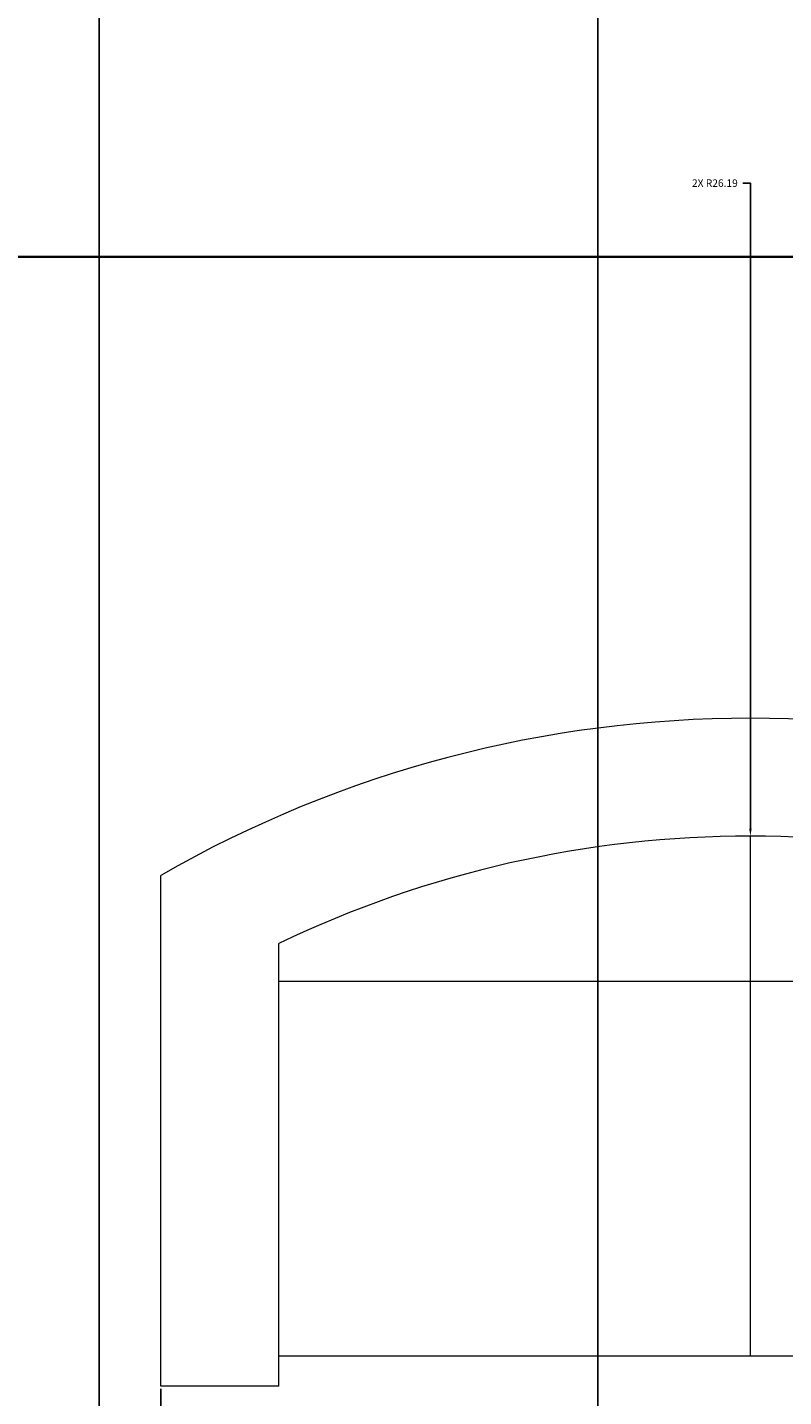
# Model space of a CAD drawing. Units: feet. Extents: x 1654 to 2985, y 1348 to 2230.
# Tile 49 of 53: x 2723 to 2741, y 1859 to 1892. Entities that reach past the tile are written whole.
import ezdxf

# ---------------------------------------------------------------- set-up
doc = ezdxf.new("R2010")
doc.units = ezdxf.units.FT
for name, color, linetype, lineweight in [('A-ANNO-DIMS', 2, 'Continuous', 18), ('A-FURN', 8, 'Continuous', 13), ('A-WALL', 7, 'Continuous', 35)]:
    doc.layers.add(name, color=color, linetype=linetype, lineweight=lineweight)
doc.styles.get("Standard").update_dxf_attribs({"font": 'arial.ttf'})
doc.dimstyles.get("Standard").update_dxf_attribs({"dimtxt": 0.18, "dimasz": 0.18, "dimexe": 0.18, "dimexo": 0.0625, "dimgap": 0.09, "dimtad": 0, "dimtih": 1, "dimtoh": 1, "dimdec": 4, "dimzin": 0, "dimdsep": 46, "dimtxsty": 'Standard', "dimcen": 0.09, "dimadec": 0, "dimazin": 0, "dimtfac": 1, "dimtdec": 4, "dimtofl": 0, "dimtmove": 0, "dimatfit": 3, "dimfxl": 1, "dimtolj": 1, "dimtzin": 0, "dimarcsym": 0})

# ---------------------------------------------------------------- blocks, each defined once
blk = doc.blocks.new('Sofa - Roundback Loveseat 5 ft.')
for p, q in [((0, -32.44198), (0, -5.99998)), ((-24, -33.99998), (-24, -11.46958)), ((24.00004, -33.99998), (24.00004, -11.46958)), ((-23.9998, -13.38178), (23.99986, -13.38178)), ((-24, -32.44198), (24.00004, -32.44198))]:
    blk.add_line(p, q)
for points in [[(-24, -33.99998), (-30, -33.99998), (-30, -7.99998)], [(30.00004, -7.99998), (30.00004, -33.99998), (24.00004, -33.99998)]]:
    blk.add_lwpolyline(points)
for centre, radius, start, end in [((0, -60.24998), 60.24998, 60.13715, 119.8628), ((0, -61.38438), 55.38444, 64.32083, 115.6792)]:
    blk.add_arc(centre, radius, start, end)
blk = doc.blocks.new('*D40')
at = {"layer": 'A-ANNO-DIMS', "color": 0, "lineweight": -2, "transparency": 16777216}
for p, q in [((2726.19, 1859.009), (2726.19, 1854.635)), ((2754.563, 1859.009), (2754.563, 1854.635)), ((2726.37, 1854.815), (2739.154, 1854.815)), ((2754.383, 1854.815), (2741.599, 1854.815))]:
    blk.add_line(p, q, dxfattribs=at)
at = {"layer": 'A-ANNO-DIMS', "color": 0, "transparency": 16777216}
for points in [[(2726.37, 1854.845), (2726.37, 1854.785), (2726.19, 1854.815)], [(2754.383, 1854.845), (2754.383, 1854.785), (2754.563, 1854.815)]]:
    blk.add_solid(points, dxfattribs=at)
at = {"layer": 'Defpoints', "color": 0, "transparency": 16777216}
for p in [(2726.19, 1859.071), (2754.563, 1859.071), (2754.563, 1854.815)]:
    blk.add_point(p, dxfattribs=at)
at = {"layer": 'A-ANNO-DIMS', "color": 0, "transparency": 16777216, "insert": (2740.376, 1854.815), "char_height": 0.18, "attachment_point": 5}
blk.add_mtext('\\A1;LOVESEAT 28 TYP.', dxfattribs=at)
blk = doc.blocks.new('*D82')
at = {"layer": 'A-ANNO-DIMS', "color": 0, "lineweight": -2, "transparency": 16777216}
for p, q in [((2652.706, 2039.192), (2652.706, 1490.625)), ((2784.706, 2039.192), (2784.706, 1490.625)), ((2652.886, 1490.805), (2718.426, 1490.805)), ((2784.526, 1490.805), (2718.985, 1490.805))]:
    blk.add_line(p, q, dxfattribs=at)
at = {"layer": 'A-ANNO-DIMS', "color": 0, "transparency": 16777216}
for points in [[(2652.886, 1490.835), (2652.886, 1490.775), (2652.706, 1490.805)], [(2784.526, 1490.835), (2784.526, 1490.775), (2784.706, 1490.805)]]:
    blk.add_solid(points, dxfattribs=at)
at = {"layer": 'Defpoints', "color": 0, "transparency": 16777216}
for p in [(2652.706, 2039.255), (2784.706, 2039.255), (2784.706, 1490.805)]:
    blk.add_point(p, dxfattribs=at)
at = {"layer": 'A-ANNO-DIMS', "color": 0, "transparency": 16777216, "insert": (2718.706, 1490.805), "char_height": 0.18, "attachment_point": 5}
blk.add_mtext('\\A1;132', dxfattribs=at)
blk = doc.blocks.new('*D87')
at = {"layer": 'A-ANNO-DIMS', "color": 0, "lineweight": -2, "transparency": 16777216}
for p, q in [((2724.706, 1565.317), (2724.706, 2149.885)), ((2736.706, 1565.317), (2736.706, 2149.885)), ((2724.886, 2149.705), (2730.496, 2149.705)), ((2736.526, 2149.705), (2730.915, 2149.705))]:
    blk.add_line(p, q, dxfattribs=at)
at = {"layer": 'A-ANNO-DIMS', "color": 0, "transparency": 16777216}
for points in [[(2724.886, 2149.735), (2724.886, 2149.675), (2724.706, 2149.705)], [(2736.526, 2149.735), (2736.526, 2149.675), (2736.706, 2149.705)]]:
    blk.add_solid(points, dxfattribs=at)
at = {"layer": 'Defpoints', "color": 0, "transparency": 16777216}
for p in [(2736.706, 2149.705), (2724.706, 1565.255), (2736.706, 1565.255)]:
    blk.add_point(p, dxfattribs=at)
at = {"layer": 'A-ANNO-DIMS', "color": 0, "transparency": 16777216, "insert": (2730.706, 2149.705), "char_height": 0.18, "attachment_point": 5}
blk.add_mtext('\\A1;12', dxfattribs=at)
blk = doc.blocks.new('*D111')
at = {"layer": 'A-ANNO-DIMS', "color": 0, "lineweight": -2, "transparency": 16777216}
for p, q in [((2740.196, 1888.027), (2740.376, 1888.027)), ((2740.376, 1888.027), (2740.376, 1872.492)), ((2740.286, 1846.122), (2740.466, 1846.122)), ((2740.376, 1846.032), (2740.376, 1846.212))]:
    blk.add_line(p, q, dxfattribs=at)
at = {"layer": 'A-ANNO-DIMS', "color": 0, "transparency": 16777216}
blk.add_solid([(2740.406, 1872.492), (2740.346, 1872.492), (2740.376, 1872.312)], dxfattribs=at)
at = {"layer": 'Defpoints', "color": 0, "transparency": 16777216}
for p in [(2740.376, 1872.312), (2740.376, 1846.122)]:
    blk.add_point(p, dxfattribs=at)
at = {"layer": 'A-ANNO-DIMS', "color": 0, "transparency": 16777216, "insert": (2739.521, 1888.027), "char_height": 0.18, "attachment_point": 5}
blk.add_mtext('\\A1;2X R26.19', dxfattribs=at)

msp = doc.modelspace()

# ---------------------------------------------------------------- linework, layer by layer
at = {"layer": 'A-WALL'}
msp.add_line((2784.7058, 1886.2549), (2652.7058, 1886.2549), dxfattribs=at)

# ---------------------------------------------------------------- block references
at = {"layer": 'A-FURN', "xscale": 0.4728872769476647, "yscale": 0.4728872769476647, "zscale": 0.4728872769476647}
msp.add_blockref('Sofa - Roundback Loveseat 5 ft.', (2740.3765, 1875.1496), dxfattribs=at)

# ---------------------------------------------------------------- dimensions: what is measured, and where the dimension line sits
at = {"layer": 'A-ANNO-DIMS'}
for base, p1, p2, picture, middle in [((2736.7058, 2149.7049), (2724.7058, 1565.2549), (2736.7058, 1565.2549), '*D87', (2730.7058, 2149.7049)), ((2784.7058, 1490.8049), (2652.7058, 2039.2549), (2784.7058, 2039.2549), '*D82', (2718.7058, 1490.8049))]:
    dim = msp.add_linear_dim(base=base, p1=p1, p2=p2, dimstyle='Standard', override={"dimdec": 0, "dimlfac": 1, "dimrnd": 0, "dimzin": 0, "dimdsep": 46, "dimlunit": 2}, dxfattribs=at)
    dim.commit()
    dim.dimension.update_dxf_attribs({"geometry": picture, "text_midpoint": middle})
dim = msp.add_radius_dim(center=(2740.3765, 1846.1218), mpoint=(2740.376, 1872.3123), text='2X <>', dimstyle='Standard', override={"dimdec": 2, "dimlfac": 1, "dimrnd": 0, "dimzin": 0, "dimdsep": 46, "dimlunit": 2}, dxfattribs=at)
dim.commit()
dim.dimension.update_dxf_attribs({"geometry": '*D111', "text_midpoint": (2739.5208, 1888.0267), "dimtype": 164})
dim = msp.add_linear_dim(base=(2754.5631, 1854.8155), p1=(2726.1899, 1859.0715), p2=(2754.5631, 1859.0715), text='LOVESEAT <> TYP.', dimstyle='Standard', override={"dimdec": 0, "dimlfac": 1, "dimrnd": 0, "dimzin": 0, "dimdsep": 46, "dimlunit": 2}, dxfattribs=at)
dim.commit()
dim.dimension.update_dxf_attribs({"geometry": '*D40', "text_midpoint": (2740.3765, 1854.8155)})

doc.saveas('drawing.dxf')
